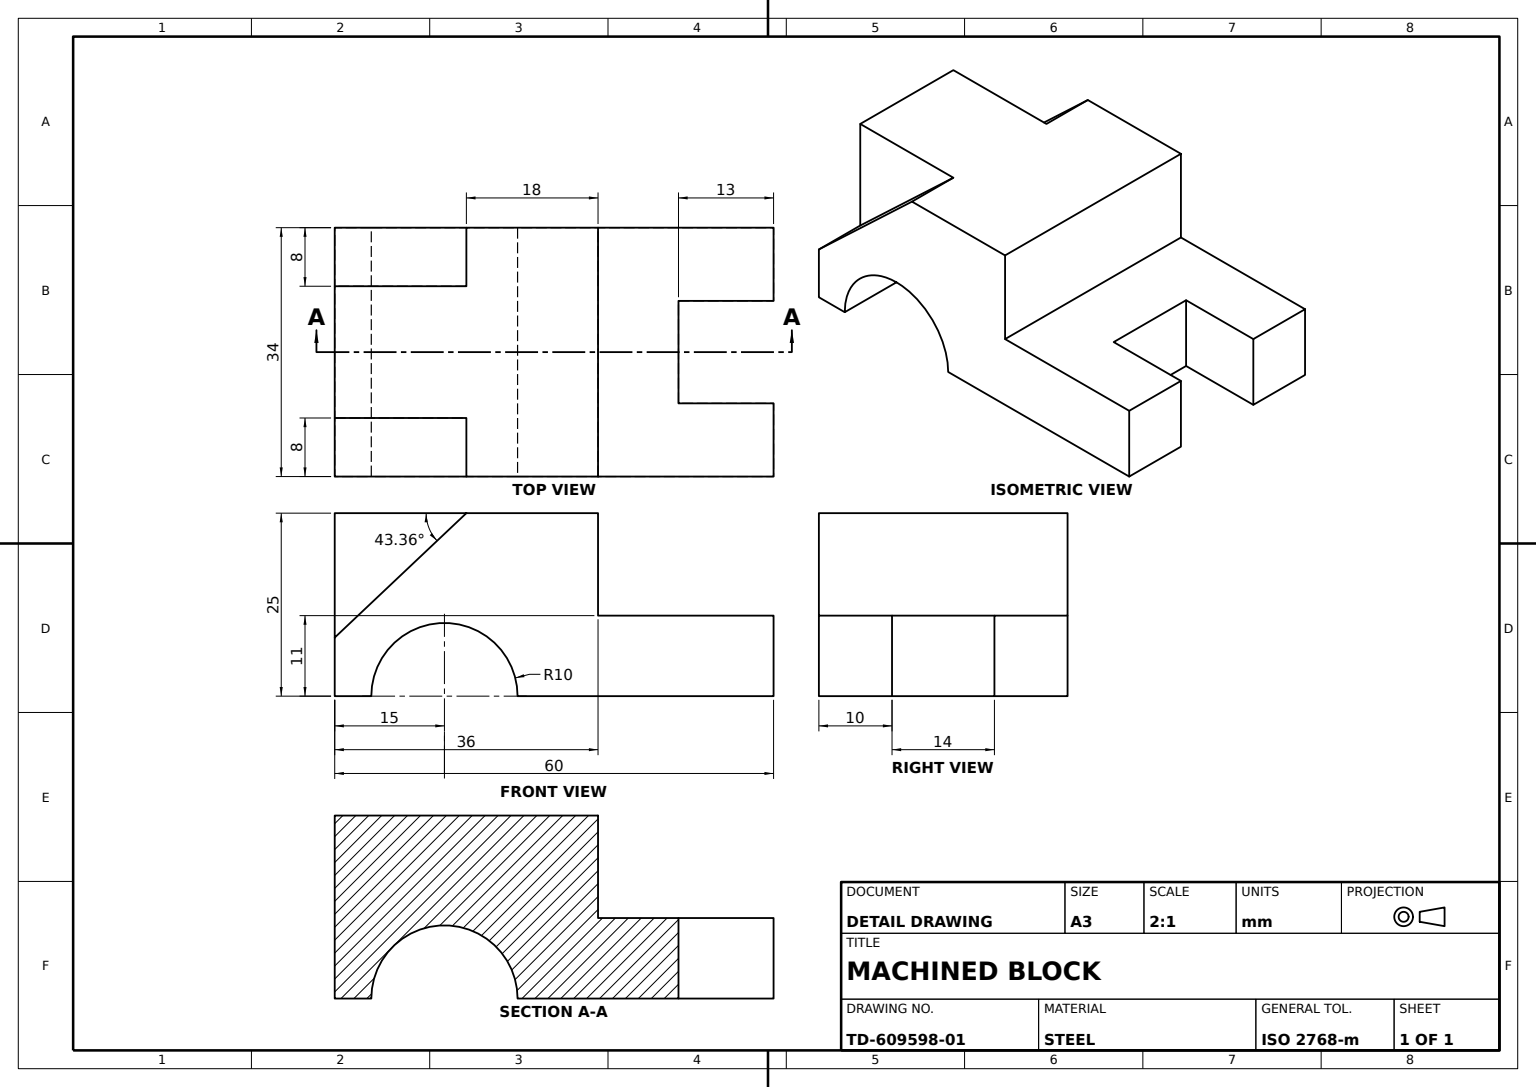
from build123d import *

# Parameters (mm, degrees)
BASE_BLOCK_DEPTH               = 17
END_SLOT_SKETCH_W              = 13
END_SLOT_SKETCH_H              = 14
END_SLOT_14X13_DEPTH           = 17
HALF_ROUND_NOTCH_R8_DEPTH      = 62.692787261
HALF_ROUND_NOTCH_R8_DEPTH_BACK = 8
SIDE_PROFILE_CUT_DEPTH         = 8


with BuildPart() as part:
    # Base Block Profile → Base Block (new, symmetric)
    with BuildSketch(Plane.XY):
        with BuildLine():
            Line((-15, 0), (-15, 25))
            Line((-15, 25), (21, 25))
            Line((21, 25), (21, 11))
            Line((21, 11), (45, 11))
            Line((45, 11), (45, 0))
            Line((45, 0), (10, 0))
            ThreePointArc((10, 0), (0, 10), (-10, 0))
            Line((-10, 0), (-15, 0))
        make_face()
    extrude(amount=BASE_BLOCK_DEPTH, both=True)

    # End Slot Sketch → End Slot 14x13 (cut, symmetric)
    with BuildSketch(Plane(origin=(0, 11, 0), x_dir=(1, 0, 0), z_dir=(0, 1, 0))):
        with Locations((38.5, 0)):
            Rectangle(END_SLOT_SKETCH_W, END_SLOT_SKETCH_H)
    extrude(amount=END_SLOT_14X13_DEPTH, both=True, mode=Mode.SUBTRACT)

    # Half-Round Notch Sketch → Half-Round Notch R8 (cut, two sides: drawn at the far end of the back side and taken through both)
    with BuildSketch(Plane.XY.offset(17).offset(-HALF_ROUND_NOTCH_R8_DEPTH_BACK)):
        Polygon((-112.94589795, -84.504459175), (-15, 8), (3, 25), (100.94589795, 117.504459175), (-84.0630204, 313.396255074), (-297.9548163, 111.387336725), align=None)
    extrude(amount=HALF_ROUND_NOTCH_R8_DEPTH + HALF_ROUND_NOTCH_R8_DEPTH_BACK, mode=Mode.SUBTRACT)

    # Side Profile Cut Sketch → Side Profile Cut (cut)
    with BuildSketch(Plane(origin=(0, 0, -17), x_dir=(-1, 0, 0), z_dir=(0, 0, -1))):
        Polygon((15, 25), (-3, 25), (15, 8), align=None)
    extrude(amount=-SIDE_PROFILE_CUT_DEPTH, mode=Mode.SUBTRACT)


solid = part.part
